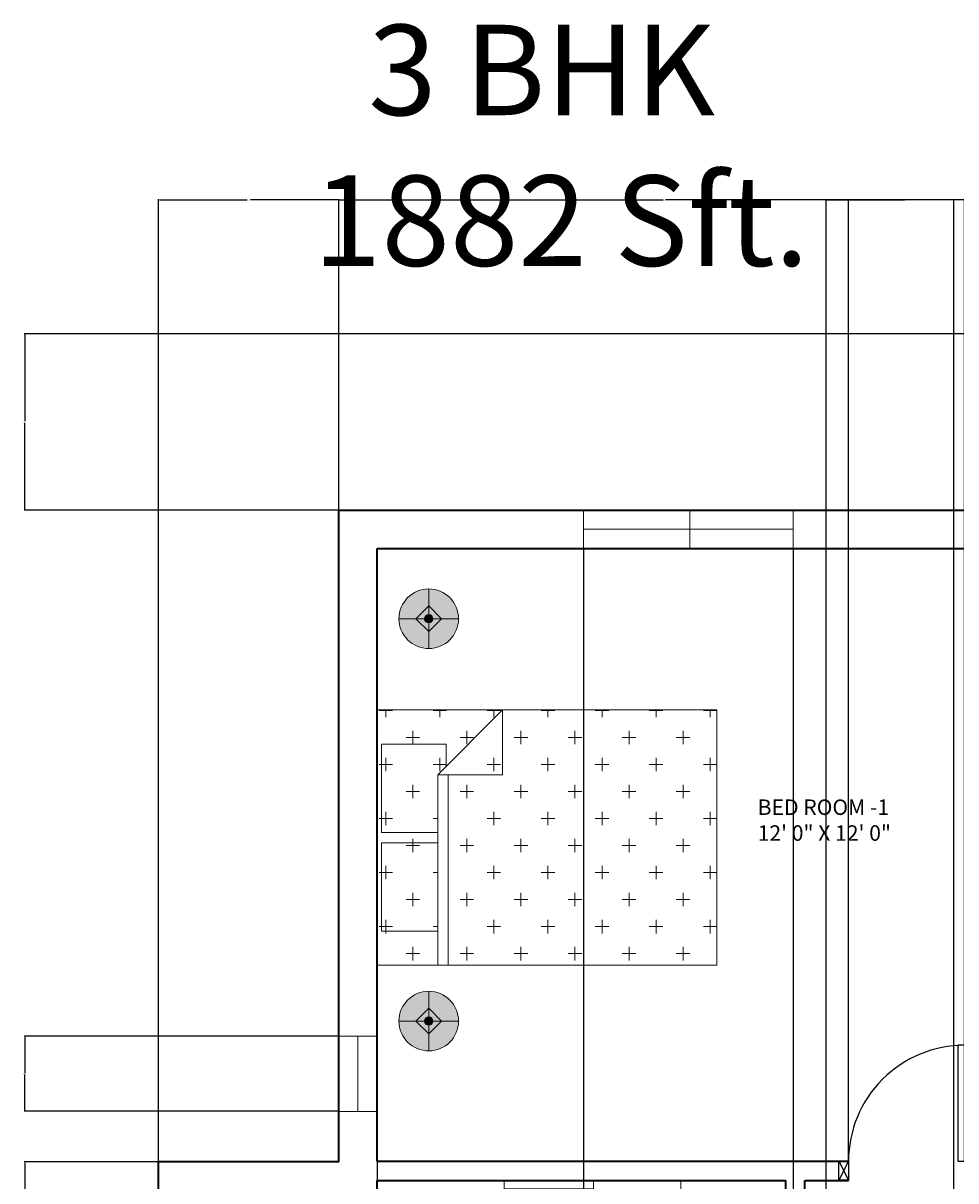
# Model space of a CAD drawing. Units: inches. Extents: x 2284228 to 3635239, y 3024422 to 8351872.
# Tile 5 of 7: x 3634669 to 3634888, y 8351600 to 8351872. Entities that reach past the tile are written whole.
import ezdxf

# ---------------------------------------------------------------- set-up
doc = ezdxf.new("R2010")
doc.units = ezdxf.units.IN
doc.linetypes.add('ACAD_ISO02W100', pattern=[15, 12, -3])
for name, color, linetype, lineweight in [('A-ANNO-DIMS', 2, 'Continuous', 18), ('A-ANNO-TEXT', 7, 'Continuous', 25), ('A-AREA-IDEN', 7, 'Continuous', 18), ('A-DOOR', 4, 'Continuous', 25), ('A-FLOR-FIXT', 9, 'Continuous', 18), ('A-FLOR-FIXT-HIDN', 9, 'ACAD_ISO02W100', 18), ('A-FURN', 8, 'Continuous', 18), ('A-FURN-PATT', 9, 'Continuous', 13), ('A-GLAZ', 4, 'Continuous', 18), ('A-WALL', 7, 'Continuous', 35)]:
    doc.layers.add(name, color=color, linetype=linetype, lineweight=lineweight)
doc.styles.get("Standard").update_dxf_attribs({"font": 'arial.ttf'})
doc.dimstyles.get("Standard").update_dxf_attribs({"dimtxt": 0.18, "dimasz": 0.18, "dimexe": 0.18, "dimexo": 0.0625, "dimgap": 0.09, "dimtad": 0, "dimtih": 1, "dimtoh": 1, "dimdec": 4, "dimzin": 0, "dimdsep": 46, "dimtxsty": 'Standard', "dimcen": 0.09, "dimadec": 0, "dimazin": 0, "dimtfac": 1, "dimtdec": 4, "dimtofl": 0, "dimtmove": 0, "dimatfit": 3, "dimfxl": 1, "dimtolj": 1, "dimtzin": 0, "dimarcsym": 0})

# ---------------------------------------------------------------- blocks, each defined once
blk = doc.blocks.new('*U9')
for p, q in [((0, 0), (0, 5)), ((30, 0), (30, 5))]:
    blk.add_line(p, q)
blk.add_lwpolyline([(0, 0), (0, -30), (1.75, -30), (1.75, 0)], close=True)
blk.add_arc((0, 0), 30, 270, 0)
blk = doc.blocks.new('Bed - Queen')
for p, q in [((0, -80.00003), (0, 0)), ((0, 0), (59.99999, 0)), ((59.99999, 0), (59.99999, -80.00003)), ((7.99999, -1.2), (28.79998, -1.2)), ((7.99999, -14.4), (7.99999, -1.2)), ((28.79998, -1.2), (28.79998, -14.4)), ((31.19999, -1.2), (51.99999, -1.2)), ((31.19999, -14.4), (31.19999, -1.2)), ((51.99999, -1.2), (51.99999, -16.4)), ((0, -14.4), (44.8, -14.4)), ((59.99999, -29.6), (44.8, -14.4)), ((44.8, -14.4), (44.8, -29.6)), ((44.8, -16.8), (0, -16.8)), ((51.99999, -16.4), (46.79936, -16.4)), ((44.8, -29.6), (59.99999, -29.6)), ((59.99999, -80.00003), (0, -80.00003))]:
    blk.add_line(p, q)
blk = doc.blocks.new('Lamp - Table')
for p, q in [((0, 7), (0, 1)), ((0, 3), (-3, 0)), ((3, 0), (0, 3)), ((-1, 0), (-7, 0)), ((-3, 0), (0, -3)), ((0, -3), (3, 0)), ((1, 0), (7, 0)), ((0, -1), (0, -7))]:
    blk.add_line(p, q)
for radius in [7, 1]:
    blk.add_circle((0, 0), radius)
blk = doc.blocks.new('Toilet - Imperial')
for p, q in [((-10, 22), (-10, 12)), ((10, 12), (10, 22)), ((-10, 21), (-7, 21)), ((-7, 20), (-10, 20)), ((-7, 21), (-7, 20)), ((10.5, 12), (-10.5, 12)), ((-10.5, 10), (-10.5, 12)), ((9, 13), (-9, 13)), ((-9, 13), (-9, 12)), ((9, 12), (9, 13)), ((10.5, 12), (10.5, 10)), ((10.5, 10), (-10.5, 10)), ((-3, 4.4065), (-3, 2)), ((-2, 2), (-2, 4.1658)), ((2, 4.1658), (2, 2)), ((3, 2), (3, 4.4065)), ((4, 2), (-4, 2)), ((-4, 2), (-4, 1)), ((4, 1), (4, 2))]:
    blk.add_line(p, q)
for points in [[(10.5, 22), (10.5, 24), (-10.5, 24), (-10.5, 22)], [(6, 0), (6, 1), (-6, 1), (-6, 0)]]:
    blk.add_lwpolyline(points, close=True)
blk.add_arc((0, 15.3333), 11.3333, 208.0725, 331.9275)
blk = doc.blocks.new('*D42')
at = {"layer": 'A-ANNO-DIMS', "color": 0, "lineweight": -2, "transparency": 16777216}
for p, q in [((3634743.25, 8351757.63), (3634743.25, 8351830.64)), ((3634743.43, 8351830.46), (3634819.47, 8351830.46)), ((3634896.07, 8351830.46), (3634820.03, 8351830.46)), ((3634896.25, 8351757.63), (3634896.25, 8351830.64))]:
    blk.add_line(p, q, dxfattribs=at)
at = {"layer": 'A-ANNO-DIMS', "color": 0, "transparency": 16777216}
for points in [[(3634743.43, 8351830.49), (3634743.43, 8351830.43), (3634743.25, 8351830.46)], [(3634896.07, 8351830.49), (3634896.07, 8351830.43), (3634896.25, 8351830.46)]]:
    blk.add_solid(points, dxfattribs=at)
at = {"layer": 'Defpoints', "color": 0, "transparency": 16777216}
for p in [(3634896.25, 8351830.46), (3634743.25, 8351757.56), (3634896.25, 8351757.56)]:
    blk.add_point(p, dxfattribs=at)
at = {"layer": 'A-ANNO-DIMS', "color": 0, "transparency": 16777216, "insert": (3634819.75, 8351830.46), "char_height": 0.18, "attachment_point": 5}
blk.add_mtext('\\A1;153', dxfattribs=at)
blk = doc.blocks.new('*D45')
at = {"layer": 'A-ANNO-DIMS', "color": 0, "lineweight": -2, "transparency": 16777216}
for p, q in [((3634896.19, 8351799.01), (3634669.29, 8351799.01)), ((3634669.47, 8351798.83), (3634669.47, 8351778.47)), ((3634669.47, 8351757.74), (3634669.47, 8351778.11)), ((3634896.19, 8351757.56), (3634669.29, 8351757.56))]:
    blk.add_line(p, q, dxfattribs=at)
at = {"layer": 'A-ANNO-DIMS', "color": 0, "transparency": 16777216}
for points in [[(3634669.44, 8351798.83), (3634669.5, 8351798.83), (3634669.47, 8351799.01)], [(3634669.44, 8351757.74), (3634669.5, 8351757.74), (3634669.47, 8351757.56)]]:
    blk.add_solid(points, dxfattribs=at)
at = {"layer": 'Defpoints', "color": 0, "transparency": 16777216}
for p in [(3634669.47, 8351799.01), (3634896.25, 8351799.01), (3634896.25, 8351757.56)]:
    blk.add_point(p, dxfattribs=at)
at = {"layer": 'A-ANNO-DIMS', "color": 0, "transparency": 16777216, "insert": (3634669.47, 8351778.29), "char_height": 0.18, "attachment_point": 5}
blk.add_mtext('\\A1;41.45', dxfattribs=at)
blk = doc.blocks.new('*D46')
at = {"layer": 'A-ANNO-DIMS', "color": 0, "lineweight": -2, "transparency": 16777216}
for p, q in [((3634700.85, 8351604.4), (3634669.29, 8351604.4)), ((3634669.47, 8351604.22), (3634669.47, 8351534.17)), ((3634669.47, 8351463.74), (3634669.47, 8351533.8)), ((3634700.85, 8351463.56), (3634669.29, 8351463.56))]:
    blk.add_line(p, q, dxfattribs=at)
at = {"layer": 'A-ANNO-DIMS', "color": 0, "transparency": 16777216}
for points in [[(3634669.44, 8351604.22), (3634669.5, 8351604.22), (3634669.47, 8351604.4)], [(3634669.44, 8351463.74), (3634669.5, 8351463.74), (3634669.47, 8351463.56)]]:
    blk.add_solid(points, dxfattribs=at)
at = {"layer": 'Defpoints', "color": 0, "transparency": 16777216}
for p in [(3634669.47, 8351604.4), (3634700.92, 8351604.4), (3634700.92, 8351463.56)]:
    blk.add_point(p, dxfattribs=at)
at = {"layer": 'A-ANNO-DIMS', "color": 0, "transparency": 16777216, "insert": (3634669.47, 8351533.98), "char_height": 0.18, "attachment_point": 5}
blk.add_mtext('\\A1;140.84', dxfattribs=at)
blk = doc.blocks.new('*D47')
at = {"layer": 'A-ANNO-DIMS', "color": 0, "lineweight": -2, "transparency": 16777216}
for p, q in [((3634700.92, 8351604.47), (3634700.92, 8351830.64)), ((3634701.1, 8351830.46), (3634721.69, 8351830.46)), ((3634743.07, 8351830.46), (3634722.48, 8351830.46)), ((3634743.25, 8351604.47), (3634743.25, 8351830.64))]:
    blk.add_line(p, q, dxfattribs=at)
at = {"layer": 'A-ANNO-DIMS', "color": 0, "transparency": 16777216}
for points in [[(3634701.1, 8351830.49), (3634701.1, 8351830.43), (3634700.92, 8351830.46)], [(3634743.07, 8351830.49), (3634743.07, 8351830.43), (3634743.25, 8351830.46)]]:
    blk.add_solid(points, dxfattribs=at)
at = {"layer": 'Defpoints', "color": 0, "transparency": 16777216}
for p in [(3634743.25, 8351830.46), (3634700.92, 8351604.4), (3634743.25, 8351604.4)]:
    blk.add_point(p, dxfattribs=at)
at = {"layer": 'A-ANNO-DIMS', "color": 0, "transparency": 16777216, "insert": (3634722.08, 8351830.46), "char_height": 0.18, "attachment_point": 5}
blk.add_mtext('\\A1;42.34', dxfattribs=at)
blk = doc.blocks.new('*D50')
at = {"layer": 'A-ANNO-DIMS', "color": 0, "lineweight": -2, "transparency": 16777216}
for p, q in [((3634800.75, 8351748.5), (3634800.75, 8351218.43)), ((3634850, 8351748.5), (3634850, 8351218.43)), ((3634800.93, 8351218.61), (3634824.98, 8351218.61)), ((3634849.82, 8351218.61), (3634825.77, 8351218.61))]:
    blk.add_line(p, q, dxfattribs=at)
at = {"layer": 'A-ANNO-DIMS', "color": 0, "transparency": 16777216}
for points in [[(3634800.93, 8351218.64), (3634800.93, 8351218.58), (3634800.75, 8351218.61)], [(3634849.82, 8351218.64), (3634849.82, 8351218.58), (3634850, 8351218.61)]]:
    blk.add_solid(points, dxfattribs=at)
at = {"layer": 'Defpoints', "color": 0, "transparency": 16777216}
for p in [(3634800.75, 8351748.56), (3634850, 8351748.56), (3634850, 8351218.61)]:
    blk.add_point(p, dxfattribs=at)
at = {"layer": 'A-ANNO-DIMS', "color": 0, "transparency": 16777216, "insert": (3634825.37, 8351218.61), "char_height": 0.18, "attachment_point": 5}
blk.add_mtext('\\A1;49.25', dxfattribs=at)
blk = doc.blocks.new('*D51')
at = {"layer": 'A-ANNO-DIMS', "color": 0, "lineweight": -2, "transparency": 16777216}
for p, q in [((3634752.25, 8351748.5), (3634752.25, 8351218.43)), ((3634800.75, 8351748.5), (3634800.75, 8351218.43)), ((3634752.43, 8351218.61), (3634776.1, 8351218.61)), ((3634800.57, 8351218.61), (3634776.9, 8351218.61))]:
    blk.add_line(p, q, dxfattribs=at)
at = {"layer": 'A-ANNO-DIMS', "color": 0, "transparency": 16777216}
for points in [[(3634752.43, 8351218.64), (3634752.43, 8351218.58), (3634752.25, 8351218.61)], [(3634800.57, 8351218.64), (3634800.57, 8351218.58), (3634800.75, 8351218.61)]]:
    blk.add_solid(points, dxfattribs=at)
at = {"layer": 'Defpoints', "color": 0, "transparency": 16777216}
for p in [(3634752.25, 8351748.56), (3634800.75, 8351748.56), (3634800.75, 8351218.61)]:
    blk.add_point(p, dxfattribs=at)
at = {"layer": 'A-ANNO-DIMS', "color": 0, "transparency": 16777216, "insert": (3634776.5, 8351218.61), "char_height": 0.18, "attachment_point": 5}
blk.add_mtext('\\A1;48.49', dxfattribs=at)
blk = doc.blocks.new('*D55')
at = {"layer": 'A-ANNO-DIMS', "color": 0, "lineweight": -2, "transparency": 16777216}
for p, q in [((3634863.01, 8351604.61), (3634863.01, 8351830.64)), ((3634863.19, 8351830.46), (3634876.18, 8351830.46)), ((3634890.1, 8351830.46), (3634877.11, 8351830.46)), ((3634890.28, 8351604.61), (3634890.28, 8351830.64))]:
    blk.add_line(p, q, dxfattribs=at)
at = {"layer": 'A-ANNO-DIMS', "color": 0, "transparency": 16777216}
for points in [[(3634863.19, 8351830.49), (3634863.19, 8351830.43), (3634863.01, 8351830.46)], [(3634890.1, 8351830.49), (3634890.1, 8351830.43), (3634890.28, 8351830.46)]]:
    blk.add_solid(points, dxfattribs=at)
at = {"layer": 'Defpoints', "color": 0, "transparency": 16777216}
for p in [(3634890.28, 8351830.46), (3634863.01, 8351604.55), (3634890.28, 8351604.55)]:
    blk.add_point(p, dxfattribs=at)
at = {"layer": 'A-ANNO-DIMS', "color": 0, "transparency": 16777216, "insert": (3634876.64, 8351830.46), "char_height": 0.18, "attachment_point": 5}
blk.add_mtext('\\A1;27.265', dxfattribs=at)
blk = doc.blocks.new('*D68')
at = {"layer": 'A-ANNO-DIMS', "color": 0, "lineweight": -2, "transparency": 16777216}
for p, q in [((3634743.19, 8351633.93), (3634669.29, 8351633.93)), ((3634669.47, 8351633.75), (3634669.47, 8351625.29)), ((3634669.47, 8351616.47), (3634669.47, 8351624.93)), ((3634743.19, 8351616.29), (3634669.29, 8351616.29))]:
    blk.add_line(p, q, dxfattribs=at)
at = {"layer": 'A-ANNO-DIMS', "color": 0, "transparency": 16777216}
for points in [[(3634669.44, 8351633.75), (3634669.5, 8351633.75), (3634669.47, 8351633.93)], [(3634669.44, 8351616.47), (3634669.5, 8351616.47), (3634669.47, 8351616.29)]]:
    blk.add_solid(points, dxfattribs=at)
at = {"layer": 'Defpoints', "color": 0, "transparency": 16777216}
for p in [(3634669.47, 8351633.93), (3634743.25, 8351633.93), (3634743.25, 8351616.29)]:
    blk.add_point(p, dxfattribs=at)
at = {"layer": 'A-ANNO-DIMS', "color": 0, "transparency": 16777216, "insert": (3634669.47, 8351625.11), "char_height": 0.18, "attachment_point": 5}
blk.add_mtext('\\A1;17.645', dxfattribs=at)
blk = doc.blocks.new('*D75')
at = {"layer": 'A-ANNO-DIMS', "color": 0, "lineweight": -2, "transparency": 16777216}
for p, q in [((3634857.77, 8351463.63), (3634857.77, 8351830.64)), ((3634857.95, 8351830.46), (3634872.56, 8351830.46)), ((3634887.59, 8351830.46), (3634872.99, 8351830.46)), ((3634887.77, 8351463.63), (3634887.77, 8351830.64))]:
    blk.add_line(p, q, dxfattribs=at)
at = {"layer": 'A-ANNO-DIMS', "color": 0, "transparency": 16777216}
for points in [[(3634857.95, 8351830.49), (3634857.95, 8351830.43), (3634857.77, 8351830.46)], [(3634887.59, 8351830.49), (3634887.59, 8351830.43), (3634887.77, 8351830.46)]]:
    blk.add_solid(points, dxfattribs=at)
at = {"layer": 'Defpoints', "color": 0, "transparency": 16777216}
for p in [(3634887.77, 8351830.46), (3634857.77, 8351463.56), (3634887.77, 8351463.56)]:
    blk.add_point(p, dxfattribs=at)
at = {"layer": 'A-ANNO-DIMS', "color": 0, "transparency": 16777216, "insert": (3634872.77, 8351830.46), "char_height": 0.18, "attachment_point": 5}
blk.add_mtext('\\A1;30', dxfattribs=at)

msp = doc.modelspace()

# ---------------------------------------------------------------- hatches: boundary and pattern name
at = {"layer": 'A-FURN-PATT'}
h = msp.add_hatch(color=256, dxfattribs=at)
h.dxf.hatch_style = 1
h.paths.add_polyline_path([(3634764.381, 8351729.0528), (3634761.381, 8351732.0528), (3634757.381, 8351732.0528, 0.41421356), (3634764.381, 8351725.0528)])
h.paths.add_polyline_path([(3634764.381, 8351735.0528), (3634764.381, 8351739.0528, 0.41421356), (3634757.381, 8351732.0528), (3634761.381, 8351732.0528)])
h.paths.add_polyline_path([(3634764.381, 8351739.0528), (3634764.381, 8351735.0528), (3634767.381, 8351732.0528), (3634771.381, 8351732.0528, 0.41421356)])
h.paths.add_polyline_path([(3634771.381, 8351732.0528), (3634767.381, 8351732.0528), (3634764.381, 8351729.0528), (3634764.381, 8351725.0528, 0.41421356)])
h = msp.add_hatch(color=256, dxfattribs=at)
h.dxf.hatch_style = 1
h.paths.add_polyline_path([(3634764.381, 8351735.0528), (3634761.381, 8351732.0528), (3634763.381, 8351732.0528, -0.41421356), (3634764.381, 8351733.0528)])
h.paths.add_polyline_path([(3634764.381, 8351735.0528), (3634764.381, 8351733.0528, -0.41421356), (3634765.381, 8351732.0528), (3634767.381, 8351732.0528)])
h.paths.add_polyline_path([(3634767.381, 8351732.0528), (3634765.381, 8351732.0528, -0.41421356), (3634764.381, 8351731.0528), (3634764.381, 8351729.0528)])
h.paths.add_polyline_path([(3634764.381, 8351731.0528, -0.41421356), (3634763.381, 8351732.0528), (3634761.381, 8351732.0528), (3634764.381, 8351729.0528)])
h = msp.add_hatch(color=256, dxfattribs=at)
h.dxf.hatch_style = 1
h.paths.add_polyline_path([(3634763.381, 8351732.0528, 1), (3634765.381, 8351732.0528, 1)])
h = msp.add_hatch(dxfattribs=at)
h.set_pattern_fill('CROSS', color=256)
h.paths.add_polyline_path([(3634832.1101, 8351710.6023), (3634781.7101, 8351710.6023), (3634781.7101, 8351695.4023), (3634768.9101, 8351695.4023), (3634768.9101, 8351650.6023), (3634832.1101, 8351650.6023)])
h.paths.add_polyline_path([(3634768.5101, 8351697.4023), (3634768.5101, 8351702.6023), (3634753.3101, 8351702.6023), (3634753.3101, 8351681.8023), (3634766.5101, 8351681.8023), (3634766.5101, 8351695.4023)], flags=17)
h.paths.add_polyline_path([(3634766.5101, 8351679.4023), (3634753.3101, 8351679.4023), (3634753.3101, 8351658.6023), (3634766.5101, 8351658.6023)], flags=17)
h.paths.add_polyline_path([(3634781.7101, 8351710.6023), (3634752.2525, 8351710.6023), (3634752.2525, 8351650.6023), (3634766.5101, 8351650.6023), (3634766.5101, 8351658.6023), (3634753.3101, 8351658.6023), (3634753.3101, 8351679.4023), (3634766.5101, 8351679.4023), (3634766.5101, 8351681.8023), (3634753.3101, 8351681.8023), (3634753.3101, 8351702.6023), (3634768.5101, 8351702.6023), (3634768.5101, 8351697.4023)])
h.paths.add_polyline_path([(3634781.7101, 8351710.6023), (3634766.5101, 8351695.4023), (3634781.7101, 8351695.4023)], flags=17)
h = msp.add_hatch(color=256, dxfattribs=at)
h.dxf.hatch_style = 1
h.paths.add_polyline_path([(3634761.381, 8351637.5022), (3634757.381, 8351637.5022, 0.41421356), (3634764.381, 8351630.5022), (3634764.381, 8351634.5022)])
h.paths.add_polyline_path([(3634764.381, 8351644.5022, 0.41421356), (3634757.381, 8351637.5022), (3634761.381, 8351637.5022), (3634764.381, 8351640.5022)])
h.paths.add_polyline_path([(3634764.381, 8351644.5022), (3634764.381, 8351640.5022), (3634767.381, 8351637.5022), (3634771.381, 8351637.5022, 0.41421356)])
h.paths.add_polyline_path([(3634771.381, 8351637.5022), (3634767.381, 8351637.5022), (3634764.381, 8351634.5022), (3634764.381, 8351630.5022, 0.41421356)])
h = msp.add_hatch(color=256, dxfattribs=at)
h.dxf.hatch_style = 1
h.paths.add_polyline_path([(3634764.381, 8351640.5022), (3634764.381, 8351638.5022, -0.41421356), (3634765.381, 8351637.5022), (3634767.381, 8351637.5022)])
h.paths.add_polyline_path([(3634764.381, 8351640.5022), (3634761.381, 8351637.5022), (3634763.381, 8351637.5022, -0.41421356), (3634764.381, 8351638.5022)])
h.paths.add_polyline_path([(3634764.381, 8351636.5022, -0.41421356), (3634763.381, 8351637.5022), (3634761.381, 8351637.5022), (3634764.381, 8351634.5022)])
h.paths.add_polyline_path([(3634767.381, 8351637.5022), (3634765.381, 8351637.5022, -0.41421356), (3634764.381, 8351636.5022), (3634764.381, 8351634.5022)])
h = msp.add_hatch(color=256, dxfattribs=at)
h.dxf.hatch_style = 1
h.paths.add_polyline_path([(3634765.381, 8351637.5022, 1), (3634763.381, 8351637.5022, 1)])

# ---------------------------------------------------------------- linework, layer by layer
at = {"layer": 'A-DOOR'}
for p, q in [((3634860.7653, 8351600.0909), (3634860.7653, 8351604.5909)), ((3634860.7653, 8351604.5909), (3634863.034, 8351600.0909)), ((3634863.034, 8351604.5909), (3634860.7653, 8351600.0909)), ((3634863.034, 8351604.5909), (3634860.7653, 8351604.5909)), ((3634863.034, 8351604.5909), (3634863.034, 8351600.0909)), ((3634863.034, 8351600.0909), (3634860.7653, 8351600.0909))]:
    msp.add_line(p, q, dxfattribs=at)
at = {"layer": 'A-FLOR-FIXT-HIDN'}
msp.add_line((3634823.6028, 8351600.0627), (3634823.6028, 8351563.6068), dxfattribs=at)
at = {"layer": 'A-GLAZ'}
for p, q in [((3634800.7459, 8351757.5627), (3634800.7459, 8351748.5627)), ((3634825.7426, 8351757.5627), (3634825.7426, 8351748.5627)), ((3634850.0004, 8351757.5627), (3634850.0004, 8351748.5627)), ((3634800.7459, 8351753.0627), (3634825.7426, 8351753.0627)), ((3634825.7426, 8351753.0627), (3634850.0004, 8351753.0627)), ((3634743.2525, 8351633.9331), (3634752.2525, 8351633.9331)), ((3634747.7525, 8351633.9331), (3634747.7525, 8351616.2882)), ((3634743.2525, 8351616.2882), (3634752.2525, 8351616.2882))]:
    msp.add_line(p, q, dxfattribs=at)
at = {"layer": 'A-WALL'}
for p, q in [((3634743.2525, 8351757.5627), (3634896.2525, 8351757.5627)), ((3634743.2525, 8351604.405), (3634743.2525, 8351757.5627)), ((3634752.2525, 8351748.5627), (3634852.7525, 8351748.5627)), ((3634752.2525, 8351604.5627), (3634752.2525, 8351748.5627)), ((3634852.7525, 8351748.5627), (3634896.2525, 8351748.5627)), ((3634700.915, 8351463.5627), (3634700.915, 8351604.405)), ((3634743.2525, 8351604.405), (3634700.915, 8351604.405)), ((3634752.2525, 8351604.5627), (3634848.2525, 8351604.5627)), ((3634752.2525, 8351604.5627), (3634848.2525, 8351604.5627)), ((3634848.2525, 8351604.5627), (3634863.034, 8351604.5627)), ((3634852.7525, 8351604.5627), (3634863.034, 8351604.5627)), ((3634752.2525, 8351600.0627), (3634848.2525, 8351600.0627)), ((3634752.2525, 8351528.0627), (3634752.2525, 8351600.0627)), ((3634848.2525, 8351528.0627), (3634848.2525, 8351600.0627)), ((3634848.2525, 8351528.0627), (3634848.2525, 8351600.0627)), ((3634852.7525, 8351463.5627), (3634852.7525, 8351600.0627)), ((3634852.7525, 8351600.0627), (3634863.0118, 8351600.0627))]:
    msp.add_line(p, q, dxfattribs=at)

# ---------------------------------------------------------------- block references
at = {"layer": 'A-DOOR', "xscale": 0.9088208868574007, "yscale": 0.9088208868574007, "zscale": 0.9088208868574007, "rotation": 180}
msp.add_blockref('*U9', (3634890.2764, 8351604.5487), dxfattribs=at)
at = {"layer": 'A-FLOR-FIXT'}
msp.add_blockref('Toilet - Imperial', (3634792.6326, 8351576.0627), dxfattribs=at)
at = {"layer": 'A-FURN'}
for p in [(3634764.381, 8351732.0528), (3634764.381, 8351637.5022)]:
    msp.add_blockref('Lamp - Table', p, dxfattribs=at)
at = {"layer": 'A-FURN', "rotation": 90}
msp.add_blockref('Bed - Queen', (3634752.1101, 8351650.6023), dxfattribs=at)

# ---------------------------------------------------------------- texts
at = {"layer": 'A-ANNO-TEXT', "insert": (3634711.2167, 8351871.6295), "char_height": 21.247108, "attachment_point": 1}
msp.add_mtext_dynamic_manual_height_columns('      3 BHK \\P    1882 Sft.', width=2288.364791, gutter_width=106.2355, heights=[0], dxfattribs=at)
at = {"layer": 'A-AREA-IDEN', "insert": (3634834.985, 8351689.579), "char_height": 3.642437, "attachment_point": 1}
msp.add_mtext_dynamic_manual_height_columns('      BED ROOM -1\\P      12\' 0" X 12\' 0"', width=222.201216, gutter_width=18.2122, heights=[0], dxfattribs=at)

# ---------------------------------------------------------------- dimensions: what is measured, and where the dimension line sits
at = {"layer": 'A-ANNO-DIMS'}
for base, p1, p2, override, picture, middle in [((3634743.2525, 8351830.4618), (3634700.915, 8351604.405), (3634743.2525, 8351604.405), {"dimdec": 2, "dimlfac": 1, "dimrnd": 0, "dimzin": 0, "dimdsep": 46, "dimlunit": 2}, '*D47', (3634722.0837, 8351830.4618)), ((3634896.2525, 8351830.4618), (3634743.2525, 8351757.5627), (3634896.2525, 8351757.5627), {"dimdec": 0, "dimlfac": 1, "dimrnd": 0, "dimzin": 0, "dimdsep": 46, "dimlunit": 2}, '*D42', (3634819.7525, 8351830.4618)), ((3634887.7742, 8351830.4618), (3634857.7742, 8351463.5627), (3634887.7742, 8351463.5627), {"dimdec": 0, "dimlfac": 1, "dimrnd": 0, "dimzin": 0, "dimdsep": 46, "dimlunit": 2}, '*D75', (3634872.7742, 8351830.4618)), ((3634890.2764, 8351830.4618), (3634863.0118, 8351604.5487), (3634890.2764, 8351604.5487), {"dimdec": 3, "dimlfac": 1, "dimrnd": 0, "dimzin": 0, "dimdsep": 46, "dimlunit": 2}, '*D55', (3634876.6441, 8351830.4618)), ((3634800.7459, 8351218.6127), (3634752.2525, 8351748.5627), (3634800.7459, 8351748.5627), {"dimdec": 2, "dimlfac": 1, "dimrnd": 0, "dimzin": 0, "dimdsep": 46, "dimlunit": 2}, '*D51', (3634776.4992, 8351218.6127)), ((3634850.0004, 8351218.6127), (3634800.7459, 8351748.5627), (3634850.0004, 8351748.5627), {"dimdec": 2, "dimlfac": 1, "dimrnd": 0, "dimzin": 0, "dimdsep": 46, "dimlunit": 2}, '*D50', (3634825.3732, 8351218.6127))]:
    dim = msp.add_linear_dim(base=base, p1=p1, p2=p2, dimstyle='Standard', override=override, dxfattribs=at)
    dim.commit()
    dim.dimension.update_dxf_attribs({"geometry": picture, "text_midpoint": middle})
for base, p1, p2, override, picture, middle in [((3634669.465, 8351799.0118), (3634896.2525, 8351757.5627), (3634896.2525, 8351799.0118), {"dimdec": 2, "dimlfac": 1, "dimrnd": 0, "dimzin": 0, "dimdsep": 46, "dimlunit": 2}, '*D45', (3634669.465, 8351778.2872)), ((3634669.465, 8351633.9331), (3634743.2525, 8351616.2882), (3634743.2525, 8351633.9331), {"dimdec": 3, "dimlfac": 1, "dimrnd": 0, "dimzin": 0, "dimdsep": 46, "dimlunit": 2}, '*D68', (3634669.465, 8351625.1106)), ((3634669.465, 8351604.405), (3634700.915, 8351463.5627), (3634700.915, 8351604.405), {"dimdec": 2, "dimlfac": 1, "dimrnd": 0, "dimzin": 0, "dimdsep": 46, "dimlunit": 2}, '*D46', (3634669.465, 8351533.9838))]:
    dim = msp.add_linear_dim(base=base, p1=p1, p2=p2, angle=90, dimstyle='Standard', override=override, dxfattribs=at)
    dim.commit()
    dim.dimension.update_dxf_attribs({"geometry": picture, "text_midpoint": middle})

doc.saveas('drawing.dxf')
